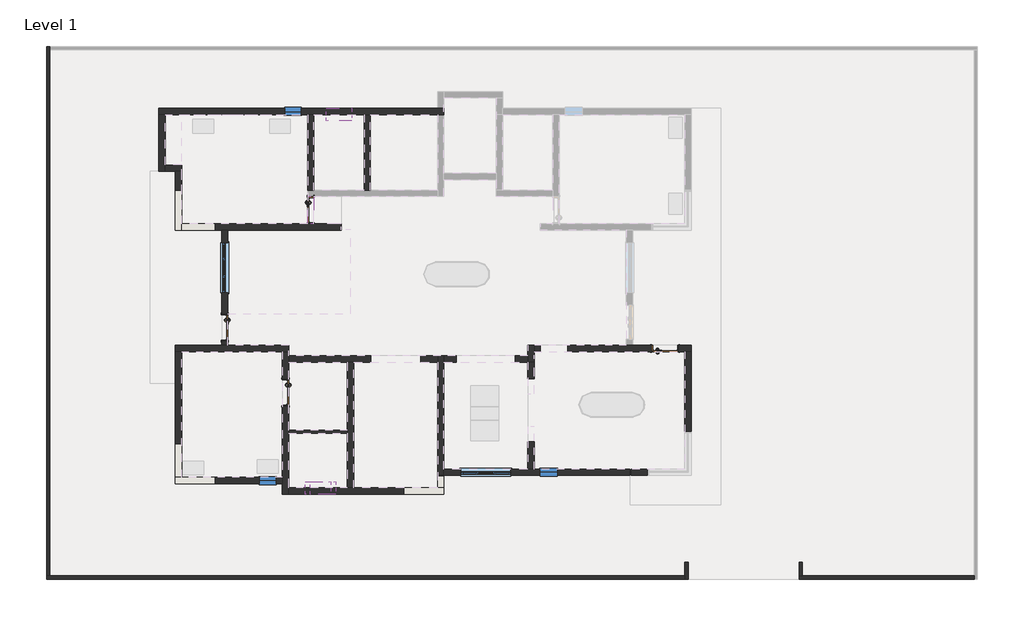
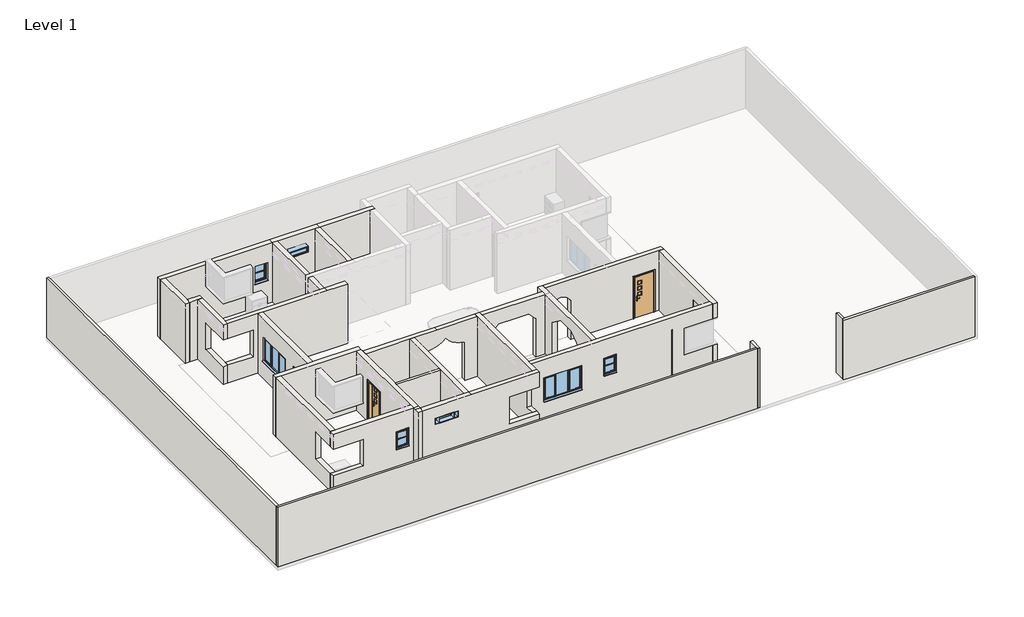
# One storey, part 1 of 2: 29 walls, 8 windows, 4 doors.
"""IFC4 building model written with IfcOpenShell, lengths in millimetres."""

from ifc_helpers import new_model, si_unit, point, frame, frame_2d, origin, origin_with_axes, place, context, project, spatial, polyline, circle_curve, trimmed, segment, composite_curve, outline, extrude, faceted_brep, transform, mapped, element, save
from ifc_brep_helpers import plane_surface, cylinder_surface, revolved_surface, advanced_brep
from components import door_3dbecc4b, door_cca51ba5, fixed_ven_3_x1_1ea7015b, windows_sgl_swept_head_window_2_x3_cc7253b0, windows_tpl_plain_window_6_x4_c25596e0

model = new_model("IFC4")

# Units and contexts
model_context = context("Model", 3, world=origin())
ifc_project = project(units=[si_unit("LENGTHUNIT", "METRE", prefix="MILLI")], contexts=[model_context])

# Site, building, storey
site = spatial("IfcSite", under=ifc_project)
building = spatial("IfcBuilding", under=site)
storey = spatial("IfcBuildingStorey", under=building, Name="Level 1", Elevation=0.0)

# Doors
placement = place(None, origin())
door_shape = door_3dbecc4b(model_context)
element("IfcDoor", 1, ObjectType="Doors_IntSgl_4 : Internal Door 3'3\"X7'", at=placement, inside=storey, context=model_context, shape_type="MappedRepresentation", body=[
    mapped(door_shape, transform((-5312.0457903, -91.9864583, 0.0), x_axis=(0.0, -1.0, 0.0), y_axis=(1.0, 0.0, 0.0), z_axis=(0.0, 0.0, 1.0))),
])
element("IfcDoor", 2, ObjectType="Doors_IntSgl_4 : Internal Door 3'3\"X7'", at=placement, inside=storey, context=model_context, shape_type="MappedRepresentation", body=[
    mapped(door_shape, transform((-3102.7378503, -2454.1864583, 0.0), x_axis=(0.0, -1.0, 0.0), y_axis=(1.0, 0.0, 0.0), z_axis=(0.0, 0.0, 1.0))),
])
door_2_shape = door_cca51ba5(model_context)
element("IfcDoor", 3, ObjectType="Doors_IntSgl_4 : Internal Door 3'3\"X7'", at=placement, inside=storey, context=model_context, shape_type="MappedRepresentation", body=[
    mapped(door_2_shape, transform((-2188.3378503, 4175.2135417, 0.0), x_axis=(0.0, -1.0, 0.0), y_axis=(1.0, 0.0, 0.0), z_axis=(0.0, 0.0, 1.0))),
])
element("IfcDoor", 4, ObjectType="Doors_IntSgl_4 : Internal Door 3'3\"X7'", at=placement, inside=storey, context=model_context, shape_type="MappedRepresentation", body=[
    mapped(door_2_shape, transform((10689.4621497, -853.9864583, 0.0), x_axis=(1.0, 0.0, 0.0), y_axis=(0.0, 1.0, 0.0), z_axis=(0.0, 0.0, 1.0))),
])

# Walls
element("IfcWall", 5, ObjectType="Generic - 4.5\"", at=placement, inside=storey, context=model_context, shape_type="SweptSolid", body=[
    extrude(outline(polyline([(-854.8378503, -3940.1648645), (-2988.4378503, -3940.1648645), (-2988.4378503, -3825.8648645), (-854.8378503, -3825.8648645), (-854.8378503, -3940.1648645)])), origin_with_axes(), (0.0, 0.0, 1.0), 3048.0),
])
element("IfcWall", 6, ObjectType="Generic - 4.5\"", at=placement, inside=storey, context=model_context, shape_type="Brep", body=[
    faceted_brep([(11413.3621497, -8626.3864583, 0.0), (11413.3621497, -9121.6864583, 0.0), (11413.3621497, -9235.9864583, 0.0), (11413.3621497, -9235.9864583, 3048.0), (11413.3621497, -9121.6864583, 3048.0), (11413.3621497, -8626.3864583, 3048.0), (11527.6621497, -8626.3864583, 0.0), (11527.6621497, -8626.3864583, 3048.0), (11527.6621497, -9235.9864583, 3048.0), (11527.6621497, -9235.9864583, 0.0)], [[[0, 1, 2, 3, 4, 5]], [[6, 7, 8, 9]], [[2, 1, 0, 6, 9]], [[5, 4, 3, 8, 7]], [[0, 5, 7, 6]], [[3, 2, 9, 8]]]),
])
element("IfcWall", 7, ObjectType="Generic - 4.5\"", at=placement, inside=storey, context=model_context, shape_type="Brep", body=[
    faceted_brep([(11413.3621497, -9121.6864583, 0.0), (-11675.2378503, -9121.6864583, 0.0), (-11789.5378503, -9121.6864583, 0.0), (-11789.5378503, -9121.6864583, 3048.0), (-11675.2378503, -9121.6864583, 3048.0), (11413.3621497, -9121.6864583, 3048.0), (11413.3621497, -9235.9864583, 0.0), (11413.3621497, -9235.9864583, 3048.0), (-11789.5378503, -9235.9864583, 3048.0), (-11789.5378503, -9235.9864583, 0.0)], [[[0, 1, 2, 3, 4, 5]], [[6, 7, 8, 9]], [[2, 1, 0, 6, 9]], [[5, 4, 3, 8, 7]], [[0, 5, 7, 6]], [[3, 2, 9, 8]]]),
])
element("IfcWall", 8, ObjectType="Generic - 4.5\"", at=placement, inside=storey, context=model_context, shape_type="Brep", body=[
    faceted_brep([(-11675.2378503, -9121.6864583, 0.0), (-11675.2378503, 10004.5135417, 0.0), (-11675.2378503, 10118.8135417, 0.0), (-11675.2378503, 10118.8135417, 3048.0), (-11675.2378503, 10004.5135417, 3048.0), (-11675.2378503, -9121.6864583, 3048.0), (-11789.5378503, -9121.6864583, 0.0), (-11789.5378503, -9121.6864583, 3048.0), (-11789.5378503, 10118.8135417, 3048.0), (-11789.5378503, 10118.8135417, 0.0)], [[[0, 1, 2, 3, 4, 5]], [[6, 7, 8, 9]], [[2, 1, 0, 6, 9]], [[5, 4, 3, 8, 7]], [[0, 5, 7, 6]], [[3, 2, 9, 8]]]),
])
element("IfcWall", 9, ObjectType="Generic - 4.5\"", at=placement, inside=storey, context=model_context, shape_type="Brep", body=[
    faceted_brep([(21928.9621497, -9121.6864583, 0.0), (15680.5621497, -9121.6864583, 0.0), (15566.2621497, -9121.6864583, 0.0), (15566.2621497, -9121.6864583, 3048.0), (15680.5621497, -9121.6864583, 3048.0), (21928.9621497, -9121.6864583, 3048.0), (21928.9621497, -9235.9864583, 0.0), (21928.9621497, -9235.9864583, 3048.0), (15566.2621497, -9235.9864583, 3048.0), (15566.2621497, -9235.9864583, 0.0)], [[[0, 1, 2, 3, 4, 5]], [[6, 7, 8, 9]], [[2, 1, 0, 6, 9]], [[5, 4, 3, 8, 7]], [[0, 5, 7, 6]], [[3, 2, 9, 8]]]),
])
element("IfcWall", 10, ObjectType="Generic - 4.5\"", at=placement, inside=storey, context=model_context, shape_type="SweptSolid", body=[
    extrude(outline(polyline([(15680.5621497, -8626.3864583), (15680.5621497, -9121.6864583), (15566.2621497, -9121.6864583), (15566.2621497, -8626.3864583), (15680.5621497, -8626.3864583)])), origin_with_axes(), (0.0, 0.0, 1.0), 3048.0),
])
element("IfcWall", 11, ObjectType="Generic - 9\"", at=placement, inside=storey, context=model_context, shape_type="Brep", body=[
    faceted_brep([(-7712.8378503, 7642.3135417, 0.0), (-7484.2378503, 7642.3135417, 0.0), (-2302.6378503, 7642.3135417, 0.0), (-2074.0378503, 7642.3135417, 0.0), (-245.2378503, 7642.3135417, 0.0), (-16.6378503, 7642.3135417, 0.0), (2421.7621497, 7642.3135417, 0.0), (2650.3621497, 7642.3135417, 0.0), (2650.3621497, 7642.3135417, 3048.0), (2421.7621497, 7642.3135417, 3048.0), (-16.6378503, 7642.3135417, 3048.0), (-245.2378503, 7642.3135417, 3048.0), (-2074.0378503, 7642.3135417, 3048.0), (-2302.6378503, 7642.3135417, 3048.0), (-7484.2378503, 7642.3135417, 3048.0), (-7712.8378503, 7642.3135417, 3048.0), (-3140.8378503, 7642.3135417, 2110.0), (-2531.2378503, 7642.3135417, 2110.0), (-2531.2378503, 7642.3135417, 1195.6), (-3140.8378503, 7642.3135417, 1195.6), (-702.4378503, 7642.3135417, 2438.4), (-702.4378503, 7642.3135417, 2133.6), (-1616.8378503, 7642.3135417, 2133.6), (-1616.8378503, 7642.3135417, 2438.4), (-7712.8378503, 7870.9135417, 0.0), (-7712.8378503, 7870.9135417, 3048.0), (-2302.6378503, 7870.9135417, 3048.0), (-16.6378503, 7870.9135417, 3048.0), (2421.7621497, 7870.9135417, 3048.0), (2650.3621497, 7870.9135417, 3048.0), (2650.3621497, 7870.9135417, 0.0), (2421.7621497, 7870.9135417, 0.0), (-3140.8378503, 7870.9135417, 2110.0), (-3140.8378503, 7870.9135417, 1195.6), (-2531.2378503, 7870.9135417, 1195.6), (-2531.2378503, 7870.9135417, 2110.0), (-702.4378503, 7870.9135417, 2438.4), (-1616.8378503, 7870.9135417, 2438.4), (-1616.8378503, 7870.9135417, 2133.6), (-702.4378503, 7870.9135417, 2133.6)], [[[0, 1, 2, 3, 4, 5, 6, 7, 8, 9, 10, 11, 12, 13, 14, 15], [16, 17, 18, 19], [20, 21, 22, 23]], [[24, 25, 26, 27, 28, 29, 30, 31], [32, 33, 34, 35], [36, 37, 38, 39]], [[7, 6, 5, 4, 3, 2, 1, 0, 24, 31, 30]], [[8, 7, 30, 29]], [[0, 15, 25, 24]], [[33, 32, 16, 19]], [[34, 33, 19, 18]], [[35, 34, 18, 17]], [[32, 35, 17, 16]], [[21, 20, 36, 39]], [[22, 21, 39, 38]], [[23, 22, 38, 37]], [[20, 23, 37, 36]], [[10, 9, 8, 29, 28, 27]], [[13, 12, 11, 10, 27, 26]], [[15, 14, 13, 26, 25]]]),
])
element("IfcWall", 12, ObjectType="Generic - 9\"", at=placement, inside=storey, context=model_context, shape_type="SweptSolid", body=[
    extrude(outline(polyline([(-2074.0378503, 7642.3135417), (-2074.0378503, 4899.1135417), (-2302.6378503, 4899.1135417), (-2302.6378503, 7642.3135417), (-2074.0378503, 7642.3135417)])), origin_with_axes(), (0.0, 0.0, 1.0), 3048.0),
])
element("IfcWall", 13, ObjectType="Generic - 9\"", at=placement, inside=storey, context=model_context, shape_type="SweptSolid", body=[
    extrude(outline(polyline([(-245.2378503, 4899.1135417), (-245.2378503, 7642.3135417), (-16.6378503, 7642.3135417), (-16.6378503, 4899.1135417), (-245.2378503, 4899.1135417)])), origin_with_axes(), (0.0, 0.0, 1.0), 3048.0),
])
element("IfcWall", 14, ObjectType="Generic - 9\"", at=placement, inside=storey, context=model_context, shape_type="Brep", body=[
    faceted_brep([(-7712.8378503, 7642.3135417, 0.0), (-7712.8378503, 5584.9135417, 0.0), (-7712.8378503, 5584.9135417, 3048.0), (-7712.8378503, 7642.3135417, 3048.0), (-7484.2378503, 7642.3135417, 0.0), (-7484.2378503, 7642.3135417, 3048.0), (-7484.2378503, 5813.5135417, 3048.0), (-7484.2378503, 5584.9135417, 3048.0), (-7484.2378503, 5584.9135417, 0.0), (-7484.2378503, 5813.5135417, 0.0)], [[[0, 1, 2, 3]], [[4, 5, 6, 7, 8, 9]], [[1, 0, 4, 9, 8]], [[0, 3, 5, 4]], [[2, 1, 8, 7]], [[3, 2, 7, 6, 5]]]),
])
element("IfcWall", 15, ObjectType="Generic - 9\"", at=placement, inside=storey, context=model_context, shape_type="Brep", body=[
    faceted_brep([(-7484.2378503, 5584.9135417, 0.0), (-7103.2378503, 5584.9135417, 0.0), (-6874.6378503, 5584.9135417, 0.0), (-6874.6378503, 5584.9135417, 3048.0), (-7103.2378503, 5584.9135417, 3048.0), (-7484.2378503, 5584.9135417, 3048.0), (-7484.2378503, 5813.5135417, 0.0), (-7484.2378503, 5813.5135417, 3048.0), (-6874.6378503, 5813.5135417, 3048.0), (-6874.6378503, 5813.5135417, 0.0)], [[[0, 1, 2, 3, 4, 5]], [[6, 7, 8, 9]], [[2, 1, 0, 6, 9]], [[0, 5, 7, 6]], [[3, 2, 9, 8]], [[5, 4, 3, 8, 7]]]),
])
element("IfcWall", 16, ObjectType="Generic - 9\"", at=placement, inside=storey, context=model_context, shape_type="Brep", body=[
    faceted_brep([(-7103.2378503, 5584.9135417, 0.0), (-7103.2378503, 3451.3135417, 0.0), (-7103.2378503, 3451.3135417, 914.4), (-7103.2378503, 4896.0865307, 914.4), (-7103.2378503, 4896.0865307, 2286.0), (-7103.2378503, 3451.3135417, 2286.0), (-7103.2378503, 3451.3135417, 3048.0), (-7103.2378503, 5584.9135417, 3048.0), (-6874.6378503, 3451.3135417, 0.0), (-6874.6378503, 3679.9135417, 0.0), (-6874.6378503, 5584.9135417, 0.0), (-6874.6378503, 5584.9135417, 3048.0), (-6874.6378503, 3679.9135417, 3048.0), (-6874.6378503, 3451.3135417, 3048.0), (-6874.6378503, 3451.3135417, 2286.0), (-6874.6378503, 3679.9135417, 2286.0), (-6874.6378503, 4896.0865307, 2286.0), (-6874.6378503, 4896.0865307, 914.4), (-6874.6378503, 3679.9135417, 914.4), (-6874.6378503, 3451.3135417, 914.4)], [[[0, 1, 2, 3, 4, 5, 6, 7]], [[8, 9, 10, 11, 12, 13, 14, 15, 16, 17, 18, 19]], [[1, 0, 10, 9, 8]], [[0, 7, 11, 10]], [[7, 6, 13, 12, 11]], [[4, 16, 15, 14, 5]], [[17, 3, 2, 19, 18]], [[16, 4, 3, 17]], [[1, 8, 19, 2]], [[13, 6, 5, 14]]]),
])
element("IfcWall", 17, ObjectType="Generic - 9\"", at=placement, inside=storey, context=model_context, shape_type="Brep", body=[
    faceted_brep([(-6874.6378503, 3451.3135417, 0.0), (-5426.3457903, 3451.3135417, 0.0), (-5197.7457903, 3451.3135417, 0.0), (-1083.4378503, 3451.3135417, 0.0), (-1083.4378503, 3451.3135417, 3048.0), (-2074.0378503, 3451.3135417, 3048.0), (-5197.7457903, 3451.3135417, 3048.0), (-5426.3457903, 3451.3135417, 3048.0), (-6874.6378503, 3451.3135417, 3048.0), (-6874.6378503, 3451.3135417, 2286.0), (-5652.1379593, 3451.3135417, 2286.0), (-5652.1379593, 3451.3135417, 914.4), (-6874.6378503, 3451.3135417, 914.4), (-1083.4378503, 3679.9135417, 0.0), (-6874.6378503, 3679.9135417, 0.0), (-6874.6378503, 3679.9135417, 914.4), (-5652.1379593, 3679.9135417, 914.4), (-5652.1379593, 3679.9135417, 2286.0), (-6874.6378503, 3679.9135417, 2286.0), (-6874.6378503, 3679.9135417, 3048.0), (-2302.6378503, 3679.9135417, 3048.0), (-2074.0378503, 3679.9135417, 3048.0), (-1083.4378503, 3679.9135417, 3048.0)], [[[0, 1, 2, 3, 4, 5, 6, 7, 8, 9, 10, 11, 12]], [[13, 14, 15, 16, 17, 18, 19, 20, 21, 22]], [[3, 2, 1, 0, 14, 13]], [[4, 3, 13, 22]], [[8, 7, 6, 5, 21, 20, 19]], [[5, 4, 22, 21]], [[17, 10, 9, 18]], [[11, 16, 15, 12]], [[10, 17, 16, 11]], [[8, 19, 18, 9]], [[14, 0, 12, 15]]]),
])
element("IfcWall", 18, ObjectType="Generic - 9\"", at=placement, inside=storey, context=model_context, shape_type="SweptSolid", body=[
    extrude(outline(polyline([(-2302.6378503, 3679.9135417), (-2302.6378503, 4670.5135417), (-2074.0378503, 4670.5135417), (-2074.0378503, 3679.9135417), (-2302.6378503, 3679.9135417)])), frame((0.0, 0.0, 2133.6), z_axis=(0.0, 0.0, 1.0), x_axis=(1.0, 0.0, 0.0)), (0.0, 0.0, 1.0), 914.4),
])
element("IfcWall", 19, ObjectType="Generic - 9\"", at=placement, inside=storey, context=model_context, shape_type="SweptSolid", body=[
    extrude(outline(polyline([(3451.3135417, 3048.0), (3451.3135417, 0.0), (403.3135417, 0.0), (403.3135417, 2133.6), (-587.2864583, 2133.6), (-587.2864583, 0.0), (-739.6864583, 0.0), (-739.6864583, 3048.0), (3451.3135417, 3048.0)]), holes=[polyline([(1164.7182292, 2110.0), (1164.7182292, 890.8), (2993.5182292, 890.8), (2993.5182292, 2110.0), (1164.7182292, 2110.0)])]), frame((-5426.3457903, 0.0, 0.0), z_axis=(1.0, 0.0, 0.0), x_axis=(0.0, 1.0, 0.0)), (0.0, 0.0, 1.0), 228.6),
])
element("IfcWall", 20, ObjectType="Generic - 9\"", at=placement, inside=storey, context=model_context, shape_type="Brep", body=[
    faceted_brep([(-7103.2378503, -968.2864583, 0.0), (-6874.6378503, -968.2864583, 0.0), (-3217.0378503, -968.2864583, 0.0), (-2988.4378503, -968.2864583, 0.0), (-2988.4378503, -968.2864583, 3048.0), (-3217.0378503, -968.2864583, 3048.0), (-6874.6378503, -968.2864583, 3048.0), (-7103.2378503, -968.2864583, 3048.0), (-7103.2378503, -739.6864583, 0.0), (-7103.2378503, -739.6864583, 3048.0), (-5426.3457903, -739.6864583, 3048.0), (-5197.7457903, -739.6864583, 3048.0), (-2988.4378503, -739.6864583, 3048.0), (-2988.4378503, -739.6864583, 0.0), (-5197.7457903, -739.6864583, 0.0), (-5426.3457903, -739.6864583, 0.0)], [[[0, 1, 2, 3, 4, 5, 6, 7]], [[8, 9, 10, 11, 12, 13, 14, 15]], [[3, 2, 1, 0, 8, 15, 14, 13]], [[4, 3, 13, 12]], [[0, 7, 9, 8]], [[7, 6, 5, 4, 12, 11, 10, 9]]]),
])
element("IfcWall", 21, ObjectType="Generic - 9\"", at=placement, inside=storey, context=model_context, shape_type="Brep", body=[
    faceted_brep([(-3217.0378503, -968.2864583, 3048.0), (-3217.0378503, -968.2864583, 0.0), (-3217.0378503, -1958.8864583, 0.0), (-3217.0378503, -1958.8864583, 2133.6), (-3217.0378503, -2949.4864583, 2133.6), (-3217.0378503, -2949.4864583, 0.0), (-3217.0378503, -5540.2864583, 0.0), (-3217.0378503, -5768.8864583, 0.0), (-3217.0378503, -6149.9648645, 0.0), (-3217.0378503, -6149.9648645, 3048.0), (-3217.0378503, -5921.3648645, 3048.0), (-3217.0378503, -5768.9648645, 3048.0), (-3217.0378503, -5540.2864583, 3048.0), (-2988.4378503, -968.2864583, 0.0), (-2988.4378503, -968.2864583, 3048.0), (-2988.4378503, -1120.6864583, 3048.0), (-2988.4378503, -1349.2864583, 3048.0), (-2988.4378503, -3825.8648645, 3048.0), (-2988.4378503, -3940.1648645, 3048.0), (-2988.4378503, -5768.9648645, 3048.0), (-2988.4378503, -5921.3648645, 3048.0), (-2988.4378503, -6149.9648645, 3048.0), (-2988.4378503, -6149.9648645, 0.0), (-2988.4378503, -5921.3648645, 0.0), (-2988.4378503, -3940.1648645, 0.0), (-2988.4378503, -3825.8648645, 0.0), (-2988.4378503, -2949.4864583, 0.0), (-2988.4378503, -2949.4864583, 2133.6), (-2988.4378503, -1958.8864583, 2133.6), (-2988.4378503, -1958.8864583, 0.0), (-2988.4378503, -1349.2864583, 0.0), (-2988.4378503, -1120.6864583, 0.0)], [[[0, 1, 2, 3, 4, 5, 6, 7, 8, 9, 10, 11, 12]], [[13, 14, 15, 16, 17, 18, 19, 20, 21, 22, 23, 24, 25, 26, 27, 28, 29, 30, 31]], [[1, 13, 31, 30, 29, 2]], [[22, 8, 7, 6, 5, 26, 25, 24, 23]], [[1, 0, 14, 13]], [[9, 8, 22, 21]], [[4, 27, 26, 5]], [[27, 4, 3, 28]], [[28, 3, 2, 29]], [[0, 12, 11, 19, 18, 17, 16, 15, 14]], [[19, 11, 10, 20]], [[9, 21, 20, 10]]]),
])
element("IfcWall", 22, ObjectType="Generic - 9\"", at=placement, inside=storey, context=model_context, shape_type="Brep", body=[
    faceted_brep([(-2988.4378503, -6149.9648645, 0.0), (2650.3621497, -6149.9648645, 0.0), (2650.3621497, -6149.9648645, 914.4), (1200.1782484, -6149.9648645, 914.4), (1200.1782484, -6149.9648645, 2286.0), (2650.3621497, -6149.9648645, 2286.0), (2650.3621497, -6149.9648645, 3048.0), (-626.2378503, -6149.9648645, 3048.0), (-2988.4378503, -6149.9648645, 3048.0), (-1286.6378503, -6149.9648645, 2133.6), (-2378.8378503, -6149.9648645, 2133.6), (-2378.8378503, -6149.9648645, 2438.4), (-1286.6378503, -6149.9648645, 2438.4), (2650.3621497, -5921.3648645, 0.0), (2421.7621497, -5921.3648645, 0.0), (-626.2378503, -5921.3648645, 0.0), (-854.8378503, -5921.3648645, 0.0), (-2988.4378503, -5921.3648645, 0.0), (-2988.4378503, -5921.3648645, 3048.0), (-854.8378503, -5921.3648645, 3048.0), (-626.2378503, -5921.3648645, 3048.0), (2421.7621497, -5921.3648645, 3048.0), (2650.3621497, -5921.3648645, 3048.0), (2650.3621497, -5921.3648645, 2286.0), (2421.7621497, -5921.3648645, 2286.0), (1200.1782484, -5921.3648645, 2286.0), (1200.1782484, -5921.3648645, 914.4), (2421.7621497, -5921.3648645, 914.4), (2650.3621497, -5921.3648645, 914.4), (-1286.6378503, -5921.3648645, 2438.4), (-2378.8378503, -5921.3648645, 2438.4), (-2378.8378503, -5921.3648645, 2133.6), (-1286.6378503, -5921.3648645, 2133.6)], [[[0, 1, 2, 3, 4, 5, 6, 7, 8], [9, 10, 11, 12]], [[13, 14, 15, 16, 17, 18, 19, 20, 21, 22, 23, 24, 25, 26, 27, 28], [29, 30, 31, 32]], [[1, 0, 17, 16, 15, 14, 13]], [[0, 8, 18, 17]], [[31, 30, 11, 10]], [[31, 10, 9, 32]], [[11, 30, 29, 12]], [[32, 9, 12, 29]], [[7, 6, 22, 21, 20]], [[8, 7, 20, 19, 18]], [[4, 25, 24, 23, 5]], [[26, 3, 2, 28, 27]], [[25, 4, 3, 26]], [[1, 13, 28, 2]], [[22, 6, 5, 23]]]),
])
element("IfcWall", 23, ObjectType="Generic - 9\"", at=placement, inside=storey, context=model_context, shape_type="Brep", body=[
    faceted_brep([(2650.3621497, -1120.6864583, 0.0), (2650.3621497, -1120.6864583, 3048.0), (2650.3621497, -1349.2864583, 3048.0), (2650.3621497, -5235.4864583, 3048.0), (2650.3621497, -5464.0864583, 3048.0), (2650.3621497, -5921.3648645, 3048.0), (2650.3621497, -5921.3648645, 2286.0), (2650.3621497, -5473.7470325, 2286.0), (2650.3621497, -5473.7470325, 914.4), (2650.3621497, -5921.3648645, 914.4), (2650.3621497, -5921.3648645, 0.0), (2650.3621497, -5467.3228508, 0.0), (2650.3621497, -5467.3228508, 2438.4), (2650.3621497, -5464.0864583, 2438.4), (2650.3621497, -5464.0864583, 0.0), (2650.3621497, -5235.4864583, 0.0), (2650.3621497, -1349.2864583, 0.0), (2421.7621497, -1120.6864583, 3048.0), (2421.7621497, -1120.6864583, 0.0), (2421.7621497, -1349.2864583, 0.0), (2421.7621497, -5464.0864583, 0.0), (2421.7621497, -5464.0864583, 2438.4), (2421.7621497, -5467.3228508, 2438.4), (2421.7621497, -5467.3228508, 0.0), (2421.7621497, -5921.3648645, 0.0), (2421.7621497, -5921.3648645, 914.4), (2421.7621497, -5473.7470325, 914.4), (2421.7621497, -5473.7470325, 2286.0), (2421.7621497, -5921.3648645, 2286.0), (2421.7621497, -5921.3648645, 3048.0), (2421.7621497, -1349.2864583, 3048.0)], [[[0, 1, 2, 3, 4, 5, 6, 7, 8, 9, 10, 11, 12, 13, 14, 15, 16]], [[17, 18, 19, 20, 21, 22, 23, 24, 25, 26, 27, 28, 29, 30]], [[10, 24, 23, 11]], [[18, 0, 16, 15, 14, 20, 19]], [[1, 0, 18, 17]], [[5, 4, 3, 2, 1, 17, 30, 29]], [[12, 22, 21, 13]], [[22, 12, 11, 23]], [[27, 7, 6, 28]], [[8, 26, 25, 9]], [[7, 27, 26, 8]], [[5, 29, 28, 6]], [[13, 21, 20, 14]], [[24, 10, 9, 25]]]),
])
element("IfcWall", 24, ObjectType="Generic - 9\"", at=placement, inside=storey, context=model_context, shape_type="AdvancedBrep", body=[
    advanced_brep(
    [(2421.7621497, -1120.6864583, 3048.0), (2421.7621497, -1120.6864583, 0.0), (1814.0713816, -1120.6864583, 0.0), (1814.0713816, -1120.6864583, 1981.2), (899.6713816, -1120.6864583, 2489.2), (-14.7286184, -1120.6864583, 2133.6), (-14.7286184, -1120.6864583, 0.0), (-2988.4378503, -1120.6864583, 0.0), (-2988.4378503, -1120.6864583, 3048.0), (478.6621497, -1120.6864583, 3048.0), (2421.7621497, -1349.2864583, 0.0), (2421.7621497, -1349.2864583, 3048.0), (478.6621497, -1349.2864583, 3048.0), (-626.2378503, -1349.2864583, 3048.0), (-854.8378503, -1349.2864583, 3048.0), (-2988.4378503, -1349.2864583, 3048.0), (-2988.4378503, -1349.2864583, 0.0), (-854.8378503, -1349.2864583, 0.0), (-626.2378503, -1349.2864583, 0.0), (-14.7286184, -1349.2864583, 0.0), (-14.7286184, -1349.2864583, 2133.6), (899.6713816, -1349.2864583, 2489.2), (1814.0713816, -1349.2864583, 1981.2), (1814.0713816, -1349.2864583, 0.0)],
    [
        (0, 1),
        (1, 2),
        (2, 3),
        (3, 4, circle_curve(frame((1884.0922514, -1120.6864583, 3184.1975656), z_axis=(0.0, 1.0, 0.0), x_axis=(1.0, 0.0, 0.0)), 1205.0336365)),
        (4, 5, circle_curve(frame((-84.7494882, -1120.6864583, 3667.110808), z_axis=(0.0, 1.0, 0.0), x_axis=(1.0, 0.0, 0.0)), 1535.1085696)),
        (5, 6),
        (6, 7),
        (7, 8),
        (8, 9),
        (9, 0),
        (10, 11),
        (11, 12),
        (12, 13),
        (13, 14),
        (14, 15),
        (15, 16),
        (16, 17),
        (17, 18),
        (18, 19),
        (19, 20),
        (20, 21, circle_curve(frame((-84.7494882, -1349.2864583, 3667.110808), z_axis=(0.0, -1.0, 0.0), x_axis=(1.0, 0.0, 0.0)), 1535.1085696)),
        (21, 22, circle_curve(frame((1884.0922514, -1349.2864583, 3184.1975656), z_axis=(0.0, -1.0, 0.0), x_axis=(1.0, 0.0, 0.0)), 1205.0336365)),
        (22, 23),
        (23, 10),
        (7, 16),
        (15, 8),
        (0, 11),
        (10, 1),
        (23, 2),
        (22, 3),
        (21, 4),
        (20, 5),
        (19, 6),
        (9, 12),
    ],
    [
        plane_surface(frame((2650.3621497, -1120.6864583, 0.0), z_axis=(0.0, 1.0, 0.0), x_axis=(-1.0, 0.0, 0.0))),
        plane_surface(frame((2650.3621497, -1349.2864583, 0.0), z_axis=(0.0, -1.0, 0.0), x_axis=(1.0, 0.0, 0.0))),
        plane_surface(frame((-2988.4378503, -739.6864583, 0.0), z_axis=(-1.0, 0.0, 0.0), x_axis=(0.0, 1.0, 0.0))),
        plane_surface(frame((2421.7621497, -6149.9648645, 0.0), z_axis=(1.0, 0.0, 0.0), x_axis=(0.0, -1.0, 0.0))),
        plane_surface(frame((2536.0621497, -1120.6864583, 0.0), z_axis=(0.0, 0.0, -1.0), x_axis=(0.0, -1.0, 0.0))),
        plane_surface(frame((1814.0713816, -1120.6864583, 0.0), z_axis=(-1.0, 0.0, 0.0), x_axis=(0.0, -1.0, 0.0))),
        cylinder_surface(frame((1884.0922514, -1349.2864583, 3184.1975656), z_axis=(0.0, 1.0, 0.0), x_axis=(1.0, 0.0, 0.0)), 1205.0336365),
        cylinder_surface(frame((-84.7494882, -1349.2864583, 3667.110808), z_axis=(0.0, 1.0, 0.0), x_axis=(1.0, 0.0, 0.0)), 1535.1085696),
        plane_surface(frame((-14.7286184, -1120.6864583, 2133.6), z_axis=(1.0, 0.0, 0.0), x_axis=(0.0, -1.0, 0.0))),
        plane_surface(frame((-14.7286184, -1120.6864583, 0.0), z_axis=(0.0, 0.0, -1.0), x_axis=(0.0, -1.0, 0.0))),
        plane_surface(frame((-16.6378503, 7870.9135417, 3048.0), z_axis=(0.0, 0.0, 1.0), x_axis=(1.0, 0.0, 0.0))),
        plane_surface(frame((478.6621497, 4899.1135417, 3048.0), z_axis=(0.0, 0.0, 1.0), x_axis=(0.0, -1.0, 0.0))),
    ],
    [
        (0, [[1, 2, 3, 4, 5, 6, 7, 8, 9, 10]]),
        (1, [[11, 12, 13, 14, 15, 16, 17, 18, 19, 20, 21, 22, 23, 24]]),
        (2, [[-8, 25, -16, 26]]),
        (3, [[27, -11, 28, -1]]),
        (4, [[-2, -28, -24, 29]]),
        (5, [[-3, -29, -23, 30]]),
        (6, [[-4, -30, -22, 31]]),
        (7, [[-5, -31, -21, 32]]),
        (8, [[-6, -32, -20, 33]]),
        (9, [[-7, -33, -19, -18, -17, -25]]),
        (10, [[-10, 34, -12, -27]]),
        (11, [[-9, -26, -15, -14, -13, -34]]),
    ],
),
])
element("IfcWall", 25, ObjectType="Generic - 9\"", at=placement, inside=storey, context=model_context, shape_type="Brep", body=[
    faceted_brep([(-854.8378503, -1349.2864583, 0.0), (-854.8378503, -3825.8648645, 0.0), (-854.8378503, -3940.1648645, 0.0), (-854.8378503, -5921.3648645, 0.0), (-854.8378503, -5921.3648645, 3048.0), (-854.8378503, -3940.1648645, 3048.0), (-854.8378503, -3825.8648645, 3048.0), (-854.8378503, -1349.2864583, 3048.0), (-626.2378503, -1349.2864583, 0.0), (-626.2378503, -1349.2864583, 3048.0), (-626.2378503, -5921.3648645, 3048.0), (-626.2378503, -5921.3648645, 0.0)], [[[0, 1, 2, 3, 4, 5, 6, 7]], [[8, 9, 10, 11]], [[3, 2, 1, 0, 8, 11]], [[4, 3, 11, 10]], [[0, 7, 9, 8]], [[7, 6, 5, 4, 10, 9]]]),
])
element("IfcWall", 26, ObjectType="Generic - 9\"", at=placement, inside=storey, context=model_context, shape_type="Brep", body=[
    faceted_brep([(-3217.0378503, -5540.2864583, 0.0), (-6874.6378503, -5540.2864583, 0.0), (-7103.2378503, -5540.2864583, 0.0), (-7103.2378503, -5540.2864583, 914.4), (-6874.6378503, -5540.2864583, 914.4), (-5652.750978, -5540.2864583, 914.4), (-5652.750978, -5540.2864583, 2286.0), (-6874.6378503, -5540.2864583, 2286.0), (-7103.2378503, -5540.2864583, 2286.0), (-7103.2378503, -5540.2864583, 3048.0), (-6874.6378503, -5540.2864583, 3048.0), (-3217.0378503, -5540.2864583, 3048.0), (-3445.6378503, -5540.2864583, 2110.0), (-4055.2378503, -5540.2864583, 2110.0), (-4055.2378503, -5540.2864583, 1195.6), (-3445.6378503, -5540.2864583, 1195.6), (-7103.2378503, -5768.8864583, 0.0), (-3217.0378503, -5768.8864583, 0.0), (-3217.0378503, -5768.8864583, 3048.0), (-7103.2378503, -5768.8864583, 3048.0), (-7103.2378503, -5768.8864583, 2286.0), (-5652.750978, -5768.8864583, 2286.0), (-5652.750978, -5768.8864583, 914.4), (-7103.2378503, -5768.8864583, 914.4), (-3445.6378503, -5768.8864583, 2110.0), (-3445.6378503, -5768.8864583, 1195.6), (-4055.2378503, -5768.8864583, 1195.6), (-4055.2378503, -5768.8864583, 2110.0)], [[[0, 1, 2, 3, 4, 5, 6, 7, 8, 9, 10, 11], [12, 13, 14, 15]], [[16, 17, 18, 19, 20, 21, 22, 23], [24, 25, 26, 27]], [[2, 1, 0, 17, 16]], [[0, 11, 18, 17]], [[25, 24, 12, 15]], [[26, 25, 15, 14]], [[27, 26, 14, 13]], [[24, 27, 13, 12]], [[11, 10, 9, 19, 18]], [[6, 21, 20, 8, 7]], [[22, 5, 4, 3, 23]], [[21, 6, 5, 22]], [[2, 16, 23, 3]], [[19, 9, 8, 20]]]),
])
element("IfcWall", 27, ObjectType="Generic - 9\"", at=placement, inside=storey, context=model_context, shape_type="SweptSolid", body=[
    extrude(outline(polyline([(-968.2864583, 0.0), (-5540.2864583, 0.0), (-5540.2864583, 914.4), (-4323.9339699, 914.4), (-4323.9339699, 2286.0), (-5540.2864583, 2286.0), (-5540.2864583, 3048.0), (-968.2864583, 3048.0), (-968.2864583, 0.0)])), frame((-7103.2378503, 0.0, 0.0), z_axis=(1.0, 0.0, 0.0), x_axis=(0.0, 1.0, 0.0)), (0.0, 0.0, 1.0), 228.6),
])
element("IfcWall", 28, ObjectType="Generic - 9\"", at=placement, inside=storey, context=model_context, shape_type="SweptSolid", body=[
    extrude(outline(polyline([(0.0, 2650.3621497), (0.0, 3107.0149713), (1981.2, 3107.0149713), (2311.4, 3437.2149713), (2311.4, 4173.8149713), (2311.4, 4910.4149713), (1981.2, 5240.6149713), (0.0, 5240.6149713), (0.0, 5698.3621497), (3048.0, 5698.3621497), (3048.0, 2650.3621497), (0.0, 2650.3621497)])), frame((0.0, -1349.2864583, 0.0), z_axis=(0.0, 1.0, 0.0), x_axis=(0.0, 0.0, 1.0)), (0.0, 0.0, 1.0), 228.6),
])
element("IfcWall", 29, ObjectType="Generic - 9\"", at=placement, inside=storey, context=model_context, shape_type="Brep", body=[
    faceted_brep([(5926.9621497, -1349.2864583, 0.0), (5926.9621497, -968.2864583, 0.0), (5926.9621497, -739.6864583, 0.0), (5926.9621497, -739.6864583, 3048.0), (5926.9621497, -968.2864583, 3048.0), (5926.9621497, -1349.2864583, 3048.0), (5698.3621497, -1349.2864583, 0.0), (5698.3621497, -1349.2864583, 3048.0), (5698.3621497, -1120.6864583, 3048.0), (5698.3621497, -739.6864583, 3048.0), (5698.3621497, -739.6864583, 0.0), (5698.3621497, -1120.6864583, 0.0)], [[[0, 1, 2, 3, 4, 5]], [[6, 7, 8, 9, 10, 11]], [[2, 1, 0, 6, 11, 10]], [[0, 5, 7, 6]], [[3, 2, 10, 9]], [[5, 4, 3, 9, 8, 7]]]),
])
element("IfcWall", 30, ObjectType="Generic - 9\"", at=placement, inside=storey, context=model_context, shape_type="AdvancedBrep", body=[
    advanced_brep(
    [(5926.9621497, -968.2864583, 0.0), (6155.5621497, -968.2864583, 0.0), (6155.5621497, -968.2864583, 1981.2), (7145.5999043, -968.2864583, 1981.2), (7145.5999043, -968.2864583, 0.0), (10194.1621497, -968.2864583, 0.0), (10194.1621497, -968.2864583, 2133.6), (11184.7621497, -968.2864583, 2133.6), (11184.7621497, -968.2864583, 0.0), (11413.3621497, -968.2864583, 0.0), (11641.9621497, -968.2864583, 0.0), (11641.9621497, -968.2864583, 3048.0), (11413.3621497, -968.2864583, 3048.0), (5926.9621497, -968.2864583, 3048.0), (6155.5621497, -739.6864583, 0.0), (5926.9621497, -739.6864583, 0.0), (5926.9621497, -739.6864583, 3048.0), (9279.7621497, -739.6864583, 3048.0), (9508.3621497, -739.6864583, 3048.0), (11641.9621497, -739.6864583, 3048.0), (11641.9621497, -739.6864583, 0.0), (11184.7621497, -739.6864583, 0.0), (11184.7621497, -739.6864583, 2133.6), (10194.1621497, -739.6864583, 2133.6), (10194.1621497, -739.6864583, 0.0), (9508.3621497, -739.6864583, 0.0), (9279.7621497, -739.6864583, 0.0), (7145.5999043, -739.6864583, 0.0), (7145.5999043, -739.6864583, 1981.2), (6155.5621497, -739.6864583, 1981.2)],
    [
        (0, 1),
        (1, 2),
        (2, 3, circle_curve(frame((6650.581027, -968.2864583, 1777.2631726), z_axis=(0.0, 1.0, 0.0), x_axis=(-1.0, 0.0, 0.0)), 535.3820304)),
        (3, 4),
        (4, 5),
        (5, 6),
        (6, 7),
        (7, 8),
        (8, 9),
        (9, 10),
        (10, 11),
        (11, 12),
        (12, 13),
        (13, 0),
        (14, 15),
        (15, 16),
        (16, 17),
        (17, 18),
        (18, 19),
        (19, 20),
        (20, 21),
        (21, 22),
        (22, 23),
        (23, 24),
        (24, 25),
        (25, 26),
        (26, 27),
        (27, 28),
        (28, 29, circle_curve(frame((6650.581027, -739.6864583, 1777.2631726), z_axis=(0.0, -1.0, 0.0), x_axis=(-1.0, 0.0, 0.0)), 535.3820304)),
        (29, 14),
        (13, 16),
        (15, 0),
        (10, 20),
        (19, 11),
        (14, 1),
        (29, 2),
        (28, 3),
        (27, 4),
        (24, 5),
        (8, 21),
        (7, 22),
        (6, 23),
    ],
    [
        plane_surface(frame((5698.3621497, -968.2864583, 0.0), z_axis=(0.0, -1.0, 0.0), x_axis=(1.0, 0.0, 0.0))),
        plane_surface(frame((5698.3621497, -739.6864583, 0.0), z_axis=(0.0, 1.0, 0.0), x_axis=(-1.0, 0.0, 0.0))),
        plane_surface(frame((5926.9621497, -1120.6864583, 0.0), z_axis=(-1.0, 0.0, 0.0), x_axis=(0.0, 1.0, 0.0))),
        plane_surface(frame((11641.9621497, -739.6864583, 0.0), z_axis=(1.0, 0.0, 0.0), x_axis=(0.0, 1.0, 0.0))),
        plane_surface(frame((5812.6621497, -968.2864583, 0.0), z_axis=(0.0, 0.0, -1.0), x_axis=(0.0, 1.0, 0.0))),
        plane_surface(frame((6155.5621497, -968.2864583, 0.0), z_axis=(1.0, 0.0, 0.0), x_axis=(0.0, 1.0, 0.0))),
        revolved_surface(polyline([(6115.1989966, -739.6864583, 1777.2631726), (6115.1989966, -968.2864583, 1777.2631726)]), (6650.581027, -739.6864583, 1777.2631726), (0.0, 1.0, 0.0)),
        plane_surface(frame((7145.5999043, -968.2864583, 1981.2), z_axis=(-1.0, 0.0, 0.0), x_axis=(0.0, 1.0, 0.0))),
        plane_surface(frame((7145.5999043, -968.2864583, 0.0), z_axis=(0.0, 0.0, -1.0), x_axis=(0.0, 1.0, 0.0))),
        plane_surface(frame((11184.7621497, -2263.6864583, 0.0), z_axis=(-1.0, 0.0, 0.0), x_axis=(0.0, 1.0, 0.0))),
        plane_surface(frame((11184.7621497, -2263.6864583, 2133.6), z_axis=(0.0, 0.0, -1.0), x_axis=(0.0, 1.0, 0.0))),
        plane_surface(frame((10194.1621497, -2263.6864583, 2133.6), z_axis=(1.0, 0.0, 0.0), x_axis=(0.0, 1.0, 0.0))),
        plane_surface(frame((-16.6378503, 7870.9135417, 3048.0), z_axis=(0.0, 0.0, 1.0), x_axis=(1.0, 0.0, 0.0))),
    ],
    [
        (0, [[1, 2, 3, 4, 5, 6, 7, 8, 9, 10, 11, 12, 13, 14]]),
        (1, [[15, 16, 17, 18, 19, 20, 21, 22, 23, 24, 25, 26, 27, 28, 29, 30]]),
        (2, [[-14, 31, -16, 32]]),
        (3, [[-11, 33, -20, 34]]),
        (4, [[-1, -32, -15, 35]]),
        (5, [[-2, -35, -30, 36]]),
        (6, [[-3, -36, -29, 37]]),
        (7, [[-4, -37, -28, 38]]),
        (8, [[-38, -27, -26, -25, 39, -5]]),
        (8, [[-33, -10, -9, 40, -21]]),
        (9, [[41, -22, -40, -8]]),
        (10, [[-41, -7, 42, -23]]),
        (11, [[-42, -6, -39, -24]]),
        (12, [[-13, -12, -34, -19, -18, -17, -31]]),
    ],
),
])
element("IfcWall", 31, ObjectType="Generic - 9\"", at=placement, inside=storey, context=model_context, shape_type="Brep", body=[
    faceted_brep([(11413.3621497, -968.2864583, 0.0), (11413.3621497, -5235.4864583, 0.0), (11413.3621497, -5464.0864583, 0.0), (11413.3621497, -5464.0864583, 914.4), (11413.3621497, -5235.4864583, 914.4), (11413.3621497, -3867.3175755, 914.4), (11413.3621497, -3867.3175755, 2286.0), (11413.3621497, -5235.4864583, 2286.0), (11413.3621497, -5464.0864583, 2286.0), (11413.3621497, -5464.0864583, 3048.0), (11413.3621497, -5235.4864583, 3048.0), (11413.3621497, -968.2864583, 3048.0), (11641.9621497, -5464.0864583, 0.0), (11641.9621497, -968.2864583, 0.0), (11641.9621497, -968.2864583, 3048.0), (11641.9621497, -5464.0864583, 3048.0), (11641.9621497, -5464.0864583, 2286.0), (11641.9621497, -3867.3175755, 2286.0), (11641.9621497, -3867.3175755, 914.4), (11641.9621497, -5464.0864583, 914.4)], [[[0, 1, 2, 3, 4, 5, 6, 7, 8, 9, 10, 11]], [[12, 13, 14, 15, 16, 17, 18, 19]], [[2, 1, 0, 13, 12]], [[0, 11, 14, 13]], [[11, 10, 9, 15, 14]], [[6, 17, 16, 8, 7]], [[18, 5, 4, 3, 19]], [[17, 6, 5, 18]], [[2, 12, 19, 3]], [[15, 9, 8, 16]]]),
])
element("IfcWall", 32, ObjectType="Generic - 9\"", at=placement, inside=storey, context=model_context, shape_type="Brep", body=[
    faceted_brep([(2650.3621497, -5235.4864583, 0.0), (2650.3621497, -5235.4864583, 3048.0), (5698.3621497, -5235.4864583, 3048.0), (5926.9621497, -5235.4864583, 3048.0), (11413.3621497, -5235.4864583, 3048.0), (11413.3621497, -5235.4864583, 2286.0), (10039.3059555, -5235.4864583, 2286.0), (10039.3059555, -5235.4864583, 914.4), (11413.3621497, -5235.4864583, 914.4), (11413.3621497, -5235.4864583, 0.0), (9458.1777679, -5235.4864583, 0.0), (9458.1777679, -5235.4864583, 2438.4), (9414.8621047, -5235.4864583, 2438.4), (9414.8621047, -5235.4864583, 0.0), (5926.9621497, -5235.4864583, 0.0), (5698.3621497, -5235.4864583, 0.0), (5088.7621497, -5235.4864583, 2110.0), (3259.9621497, -5235.4864583, 2110.0), (3259.9621497, -5235.4864583, 890.8), (5088.7621497, -5235.4864583, 890.8), (6765.1621497, -5235.4864583, 2110.0), (6155.5621497, -5235.4864583, 2110.0), (6155.5621497, -5235.4864583, 1195.6), (6765.1621497, -5235.4864583, 1195.6), (2650.3621497, -5464.0864583, 3048.0), (2650.3621497, -5464.0864583, 2438.4), (2650.3621497, -5464.0864583, 0.0), (9414.8621047, -5464.0864583, 0.0), (9414.8621047, -5464.0864583, 2438.4), (9458.1777679, -5464.0864583, 2438.4), (9458.1777679, -5464.0864583, 0.0), (11413.3621497, -5464.0864583, 0.0), (11413.3621497, -5464.0864583, 914.4), (10039.3059555, -5464.0864583, 914.4), (10039.3059555, -5464.0864583, 2286.0), (11413.3621497, -5464.0864583, 2286.0), (11413.3621497, -5464.0864583, 3048.0), (9736.9621497, -5464.0864583, 3048.0), (5088.7621497, -5464.0864583, 2110.0), (5088.7621497, -5464.0864583, 890.8), (3259.9621497, -5464.0864583, 890.8), (3259.9621497, -5464.0864583, 2110.0), (6765.1621497, -5464.0864583, 2110.0), (6765.1621497, -5464.0864583, 1195.6), (6155.5621497, -5464.0864583, 1195.6), (6155.5621497, -5464.0864583, 2110.0)], [[[0, 1, 2, 3, 4, 5, 6, 7, 8, 9, 10, 11, 12, 13, 14, 15], [16, 17, 18, 19], [20, 21, 22, 23]], [[24, 25, 26, 27, 28, 29, 30, 31, 32, 33, 34, 35, 36, 37], [38, 39, 40, 41], [42, 43, 44, 45]], [[9, 31, 30, 10]], [[26, 0, 15, 14, 13, 27]], [[39, 38, 16, 19]], [[40, 39, 19, 18]], [[41, 40, 18, 17]], [[38, 41, 17, 16]], [[43, 42, 20, 23]], [[44, 43, 23, 22]], [[45, 44, 22, 21]], [[42, 45, 21, 20]], [[4, 3, 2, 1, 24, 37, 36]], [[11, 29, 28, 12]], [[29, 11, 10, 30]], [[12, 28, 27, 13]], [[34, 6, 5, 35]], [[7, 33, 32, 8]], [[6, 34, 33, 7]], [[4, 36, 35, 5]], [[1, 0, 26, 25, 24]], [[31, 9, 8, 32]]]),
])
element("IfcWall", 33, ObjectType="Generic - 9\"", at=placement, inside=storey, context=model_context, shape_type="SweptSolid", body=[
    extrude(outline(composite_curve([segment(polyline([(-1349.2864583, 0.0), (-1959.1091371, 0.0), (-1959.1091371, 1981.2)]), True, "CONTINUOUS"), segment(trimmed(circle_curve(frame_2d((-3102.1091371, 1178.3788323)), 1396.771573), [point((-1959.1091371, 1981.2))], [point((-4245.1091371, 1981.2))], True, "CARTESIAN"), True, "CONTINUOUS"), segment(polyline([(-4245.1091371, 1981.2), (-4245.1091371, 0.0), (-5235.4864583, 0.0), (-5235.4864583, 3048.0), (-1349.2864583, 3048.0), (-1349.2864583, 0.0)]), True, "CONTINUOUS")], self_intersect=False)), frame((5698.3621497, 0.0, 0.0), z_axis=(1.0, 0.0, 0.0), x_axis=(0.0, 1.0, 0.0)), (0.0, 0.0, 1.0), 228.6),
])

# Windows
fixed_ven_3_x1_shape = fixed_ven_3_x1_1ea7015b(model_context)
element("IfcWindow", 34, ObjectType="Fixed : Ven 3'X1'", at=placement, inside=storey, context=model_context, shape_type="MappedRepresentation", body=[
    mapped(fixed_ven_3_x1_shape, transform((-1959.7378503, -6035.6648645, 0.0), x_axis=(-1.0, 0.0, 0.0), y_axis=(0.0, -1.0, 0.0), z_axis=(0.0, 0.0, 1.0))),
])
element("IfcWindow", 35, ObjectType="Fixed : Ven 3'X1'", at=placement, inside=storey, context=model_context, shape_type="MappedRepresentation", body=[
    mapped(fixed_ven_3_x1_shape, transform((-1781.9378503, -6035.6648645, 0.0), x_axis=(-1.0, 0.0, 0.0), y_axis=(0.0, -1.0, 0.0), z_axis=(0.0, 0.0, 1.0))),
])
element("IfcWindow", 36, ObjectType="Fixed : Ven 3'X1'", at=placement, inside=storey, context=model_context, shape_type="MappedRepresentation", body=[
    mapped(fixed_ven_3_x1_shape, transform((-1121.5378503, 7756.6135417, 0.0), x_axis=(1.0, 0.0, 0.0), y_axis=(0.0, 1.0, 0.0), z_axis=(0.0, 0.0, 1.0))),
])
windows_sgl_swept_head_window_2_x3_shape = windows_sgl_swept_head_window_2_x3_cc7253b0(model_context)
element("IfcWindow", 37, ObjectType="Windows_Sgl_Swept_Head : Window 2'X3'", at=placement, inside=storey, context=model_context, shape_type="MappedRepresentation", body=[
    mapped(windows_sgl_swept_head_window_2_x3_shape, transform((6460.3621497, -5341.3298904, 0.0), x_axis=(-1.0, 0.0, 0.0), y_axis=(0.0, -1.0, 0.0), z_axis=(0.0, 0.0, 1.0))),
])
element("IfcWindow", 38, ObjectType="Windows_Sgl_Swept_Head : Window 2'X3'", at=placement, inside=storey, context=model_context, shape_type="MappedRepresentation", body=[
    mapped(windows_sgl_swept_head_window_2_x3_shape, transform((-3750.4378503, -5646.1298904, 0.0), x_axis=(-1.0, 0.0, 0.0), y_axis=(0.0, -1.0, 0.0), z_axis=(0.0, 0.0, 1.0))),
])
element("IfcWindow", 39, ObjectType="Windows_Sgl_Swept_Head : Window 2'X3'", at=placement, inside=storey, context=model_context, shape_type="MappedRepresentation", body=[
    mapped(windows_sgl_swept_head_window_2_x3_shape, transform((-2836.0378503, 7748.1569739, 0.0), x_axis=(1.0, 0.0, 0.0), y_axis=(0.0, 1.0, 0.0), z_axis=(0.0, 0.0, 1.0))),
])
windows_tpl_plain_window_6_x4_shape = windows_tpl_plain_window_6_x4_c25596e0(model_context)
element("IfcWindow", 40, ObjectType="Windows_Tpl_Plain : Window 6'X4'", at=placement, inside=storey, context=model_context, shape_type="MappedRepresentation", body=[
    mapped(windows_tpl_plain_window_6_x4_shape, transform((-5303.5892224, 2658.9182292, 0.0), x_axis=(0.0, 1.0, 0.0), y_axis=(-1.0, 0.0, 0.0), z_axis=(0.0, 0.0, 1.0))),
])
element("IfcWindow", 41, ObjectType="Windows_Tpl_Plain : Window 6'X4'", at=placement, inside=storey, context=model_context, shape_type="MappedRepresentation", body=[
    mapped(windows_tpl_plain_window_6_x4_shape, transform((3594.5621497, -5341.3298904, 0.0), x_axis=(-1.0, 0.0, 0.0), y_axis=(0.0, -1.0, 0.0), z_axis=(0.0, 0.0, 1.0))),
])

save(model, "model.ifc")

# Revit data of these elements
# Type "Doors_IntSgl_4 : Internal Door 3'3\"X7'"
#   Type Mark = "13"
#   Type Comments = "Internal Single"
#   Operation = "SingleSwingRight"
#   Construction Type Id = "SGL"
#   Manufacturer = "Revit"
#   Keynote = "L20"
#   Description = "Internal Single Door"
#   Analytic Construction = "Large single-glazed windows"
#   Visual Light Transmittance = 0.9
#   VisionPanel Width = 0' - 7.28346"
#   VisionPanel Depth = 0' - 7.28346"
#   UnderCut = 0' - 0.31496"
#   Tolerance = 0' - 0.07874"
#   Thickness = 0' - 1.49606"
#   Structural Tolerance = 0' - 0.31496"
#   StopDepth = 0' - 1.25984"
#   Stop Thickness = 0' - 0.74803"
#   Stile Shutting = 0' - 6.10236"
#   Stile Top Rail = 0' - 9.84252"
#   Stile Intermediate/Frieze = 0' - 3.93701"
#   Solar Heat Gain Coefficient = 0.86
#   Rough Width = 3' - 3"
#   Rough Height = 7' - 0"
#   Heat Transfer Coefficient (U) = 0.979472 BTU/(h·ft²·°F)
#   Handle Z Distance = 3' - 3.37008"
#   Handle X Distance = 0' - 2.95276"
#   Handle Length = 1' - 1.77953"
#   Frame Thickness = 0' - 1.25984"
#   Door Panel Width = 2' - 11.69291"
#   Door Panel Thickness = 0' - 1.49606"
#   Door Panel Offset = 0' - 0"
#   Height = 7' - 0"
#   Width = 3' - 3"
#   Door Panel Height = 6' - 10.0315"
#   Architrave Setback = 0' - 0.19685"
#   Vis - Ironmongery = yes
#   Define Thermal Properties by = 1
#   Material Ironmongery = Door - Handle
#   Material Glass = Door - Glazing
#   Material Frame = Door - Frame/Mullion
#   Material Door = Door - Panel
#   Material Beading = Door - Panel
#   Material Architrave = Door - Architrave
#   Handle Style = element 386699
#   Function = (empty or 0)
#   Wall Closure = (empty or 0)
# Type "Generic - 4.5\""
#   Assembly Code = "B2010"
#   Layers, outside or top first: 0' - 4 1/2" no material (function 1)
# Type "Generic - 9\""
#   Assembly Code = "B2010"
#   Layers, outside or top first: 0' - 9" no material (function 1)
# Type "Fixed : Ven 3'X1'"
#   Type Mark = "32"
#   Construction Type Id = "GSP4R"
#   Assembly Code = "B2020100"
#   Analytic Construction = "1/8 in Pilkington single glazing"
#   Rough Width = 3' - 0"
#   Rough Height = 1' - 0"
#   Visual Light Transmittance = 0.9
#   Solar Heat Gain Coefficient = 0.78
#   Heat Transfer Coefficient (U) = 0.6496 BTU/(h·ft²·°F)
#   Height = 1' - 0"
#   Default Sill Height = 7' - 0"
#   Width = 3' - 0"
#   Window Inset = 1' - 4"
#   Define Thermal Properties by = 1
#   Glass Pane Material = Glass
#   Sash Material = Sash
#   Wall Closure = (empty or 0)
# Type "Windows_Sgl_Swept_Head : Window 2'X3'"
#   Type Mark = "31"
#   Operation = "SinglePanel"
#   Construction Type Id = "SGL"
#   Manufacturer = "Revit"
#   Keynote = "L10"
#   Analytic Construction = "Large single-glazed windows"
#   Wrap Layers (Ext) from Ext = 0' - 4.03543"
#   Wrap Layers (Int) from Ext = 0' - 6.98819"
#   Window Board Projection = 0' - 0.98425"
#   Window Board Extension = 0' - 0.98425"
#   Visual Light Transmittance = 0.9
#   Solar Heat Gain Coefficient = 0.86
#   Rough Width = 2' - 0"
#   Rough Height = 3' - 0"
#   Radius - Swept Head = 2' - 11.81102"
#   Height = 3' - 0"
#   Width = 2' - 0"
#   Heat Transfer Coefficient (U) = 0.979472 BTU/(h·ft²·°F)
#   Glazing Thickness = 0' - 0.94488"
#   FrameOffset - External = 0' - 1.9685"
#   Frame Depth = 0' - 2.55906"
#   Default Head Height = 6' - 11.07087"
#   Cill Depth = 0' - 3.44488"
#   Cavity Closer Width = 0' - 1.9685"
#   Cavity Closer Offset from Ext = 0' - 4.03543"
#   Cavity Closer Depth = 0' - 3.34646"
#   Vis - Cavity Closers = yes
#   Define Thermal Properties by = 1
#   Material Trim = Window Frame
#   Material Glass = Glass
#   Material Frame = Window Frame
#   Wall Closure = (empty or 0)
# Type "Windows_Tpl_Plain : Window 6'X4'"
#   Type Mark = "24"
#   Operation = "TriplePanelVertical"
#   Construction Type Id = "GSP4R"
#   Manufacturer = "Revit"
#   Keynote = "L10"
#   Analytic Construction = "1/8 in Pilkington single glazing"
#   Wrap Layers (Ext) from Ext = 0' - 4.03543"
#   Wrap Layers (Int) from Ext = 0' - 6.98819"
#   Window Board Projection = 0' - 0.98425"
#   Window Board Extension = 0' - 0.98425"
#   Visual Light Transmittance = 0.9
#   Solar Heat Gain Coefficient = 0.78
#   Rough Width = 6' - 0"
#   Rough Height = 4' - 0"
#   Height = 4' - 0"
#   Width = 6' - 0"
#   Heat Transfer Coefficient (U) = 0.6496 BTU/(h·ft²·°F)
#   Glazing Thickness = 0' - 0.94488"
#   FrameOffset - External = 0' - 1.9685"
#   Frame Depth = 0' - 2.55906"
#   Default Head Height = 6' - 11.07087"
#   Cill Depth = 0' - 3.44488"
#   Cavity Closer Width = 0' - 1.9685"
#   Cavity Closer Offset from Ext = 0' - 4.03543"
#   Cavity Closer Depth = 0' - 3.34646"
#   Vis - Cavity Closers = yes
#   Define Thermal Properties by = 1
#   Material Trim = Window Frame
#   Material Glass = Glass
#   Material Frame = Window Frame
#   Wall Closure = (empty or 0)
# Elements 1, 2, 3, 4 (IfcDoor, "Doors_IntSgl_4 : Internal Door 3'3\"X7'")
#   Phase Created = New Construction
#   Materials on its faces: "Door - Panel", "Door - Architrave", "Door - Handle", "Door - Frame/Mullion", "Door - Glazing"
# Element 5 (IfcWall, "Generic - 4.5\"")
#   Top Offset = 0' - 0"
#   Base Offset = 0' - 0"
#   wall height = 10' - 0"
#   Phase Created = New Construction
#   Base Constraint = Level 1
#   Top Constraint = Level 2
#   Materials on its faces: "Default Wall"
# Elements 6, 7, 8, 9, 10 (IfcWall, "Generic - 4.5\"")
#   Top Offset = 0' - 0"
#   Base Offset = 0' - 0"
#   Unconnected Height = 10' - 0"
#   wall height = 10' - 0"
#   Phase Created = New Construction
#   Base Constraint = Level 1
#   Materials on its faces: "Default Wall", "Beige Colour"
# Elements 11, 14, 15, 16, 17, 19, 20, 21, 22, 23, 26, 27, 29, 30, 31, 32 (IfcWall, "Generic - 9\"")
#   Top Offset = 0' - 0"
#   Base Offset = 0' - 0"
#   wall height = 10' - 0"
#   Phase Created = New Construction
#   Base Constraint = Level 1
#   Top Constraint = Level 2
#   Materials on its faces: "Default Wall", "Beige Colour"
# Elements 12, 13, 18, 24, 25, 28, 33 (IfcWall, "Generic - 9\"")
#   Top Offset = 0' - 0"
#   Base Offset = 0' - 0"
#   wall height = 10' - 0"
#   Phase Created = New Construction
#   Base Constraint = Level 1
#   Top Constraint = Level 2
#   Materials on its faces: "Default Wall"
# Element 34 (IfcWindow, "Fixed : Ven 3'X1'")
#   Mark = "8"
#   Phase Created = New Construction
#   Materials on its faces: "Sash", "Glass"
# Element 35 (IfcWindow, "Fixed : Ven 3'X1'")
#   Mark = "9"
#   Phase Created = New Construction
#   Materials on its faces: "Sash", "Glass"
# Element 36 (IfcWindow, "Fixed : Ven 3'X1'")
#   Mark = "10"
#   Phase Created = New Construction
#   Materials on its faces: "Sash", "Glass"
# Element 37 (IfcWindow, "Windows_Sgl_Swept_Head : Window 2'X3'")
#   Mark = "4"
#   Phase Created = New Construction
#   Materials on its faces: "Window Frame", "Glass"
# Element 38 (IfcWindow, "Windows_Sgl_Swept_Head : Window 2'X3'")
#   Mark = "5"
#   Phase Created = New Construction
#   Materials on its faces: "Window Frame", "Glass"
# Element 39 (IfcWindow, "Windows_Sgl_Swept_Head : Window 2'X3'")
#   Mark = "6"
#   Phase Created = New Construction
#   Materials on its faces: "Window Frame", "Glass"
# Element 40 (IfcWindow, "Windows_Tpl_Plain : Window 6'X4'")
#   Mark = "1"
#   Phase Created = New Construction
#   Materials on its faces: "Window Frame", "Glass"
# Element 41 (IfcWindow, "Windows_Tpl_Plain : Window 6'X4'")
#   Mark = "3"
#   Phase Created = New Construction
#   Materials on its faces: "Window Frame", "Glass"
# Materials
#   "Door - Handle": colour RGB 247 247 247, transparency 0
#   "Door - Glazing": colour RGB 0 0 255, transparency 0.75
#   "Door - Frame/Mullion": class "Wood", colour RGB 212 179 113, transparency 0
#   "Door - Panel": class "Wood", colour RGB 210 159 95, transparency 0, Cost = 0
#   "Door - Architrave": class "Wood", colour RGB 212 179 113, transparency 0
#   "Glass": class "Glass", colour RGB 0 128 192, transparency 0.75, Description = "Soda Lime Glass", Cost = 0
#   "Sash": class "Wood", colour RGB 224 178 126, transparency 0, Cost = 0
#   "Window Frame": colour RGB 249 249 249, transparency 0
#   "Default Wall": colour RGB 128 128 128, transparency 0, Cost = 0
#   "Beige Colour": class "Generic", colour RGB 120 120 120, transparency 0, Cost = 0
